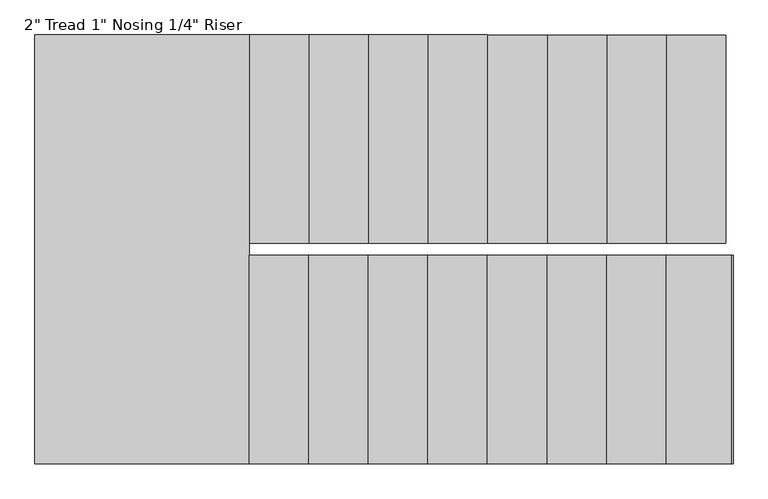
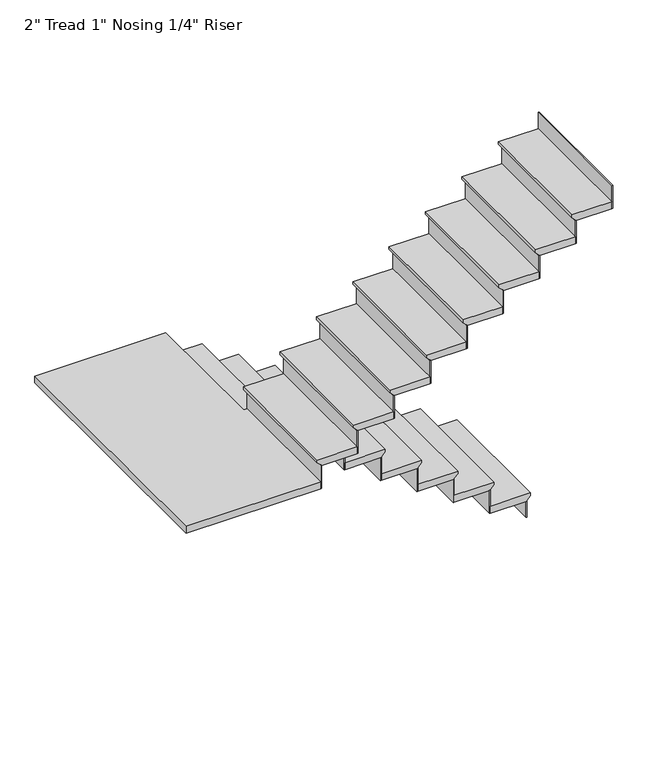
"""IFC4 building model written with IfcOpenShell, lengths in millimetres: stair flight geometry."""

from ifc_helpers import new_model, si_unit, origin, place, context, project, spatial, faceted_brep, source, transform, mapped, element, save


def stair_flight_80fd211d(model_context):
    return source(origin(), model_context, "Body", "Brep", [
        faceted_brep([(-2748.0012202, 5930.6309003, 3198.2833333), (-2748.0012202, 5930.6309003, 3217.3333333), (-2748.0012202, 5041.6309003, 3217.3333333), (-2748.0012202, 5041.6309003, 3198.2833333), (-2773.4012202, 5930.6309003, 3172.8833333), (-2773.4012202, 5041.6309003, 3172.8833333), (-3027.4012202, 5930.6309003, 3217.3333333), (-3027.4012202, 5041.6309003, 3217.3333333), (-2773.4012202, 5041.6309003, 3166.5333333), (-3027.4012202, 5041.6309003, 3166.5333333), (-3027.4012202, 5930.6309003, 3166.5333333), (-2773.4012202, 5930.6309003, 3166.5333333)], [[[0, 1, 2, 3]], [[4, 0, 3, 5]], [[2, 1, 6, 7]], [[8, 9, 10, 11]], [[2, 7, 9, 8, 5, 3]], [[8, 11, 4, 5]], [[6, 1, 0, 4, 11, 10]], [[7, 6, 10, 9]]]),
        faceted_brep([(-2773.4012202, 5930.6309003, 3166.5333333), (-2773.4012202, 5930.6309003, 3048.0), (-2779.7512202, 5930.6309003, 3048.0), (-2779.7512202, 5930.6309003, 3166.5333333), (-2773.4012202, 5041.6309003, 3166.5333333), (-2779.7512202, 5041.6309003, 3166.5333333), (-2779.7512202, 5041.6309003, 3048.0), (-2773.4012202, 5041.6309003, 3048.0)], [[[0, 1, 2, 3]], [[4, 5, 6, 7]], [[1, 0, 4, 7]], [[2, 1, 7, 6]], [[3, 2, 6, 5]], [[0, 3, 5, 4]]]),
        faceted_brep([(-3027.4012202, 5930.6309003, 3335.8666667), (-3027.4012202, 5930.6309003, 3166.5333333), (-3033.7512202, 5930.6309003, 3166.5333333), (-3033.7512202, 5930.6309003, 3335.8666667), (-3027.4012202, 5041.6309003, 3335.8666667), (-3033.7512202, 5041.6309003, 3335.8666667), (-3033.7512202, 5041.6309003, 3166.5333333), (-3027.4012202, 5041.6309003, 3166.5333333)], [[[0, 1, 2, 3]], [[4, 5, 6, 7]], [[1, 0, 4, 7]], [[2, 1, 7, 6]], [[3, 2, 6, 5]], [[0, 3, 5, 4]]]),
        faceted_brep([(-3002.0012202, 5041.6309003, 3386.6666667), (-3002.0012202, 5930.6309003, 3386.6666667), (-3281.4012202, 5930.6309003, 3386.6666667), (-3281.4012202, 5041.6309003, 3386.6666667), (-3027.4012202, 5041.6309003, 3335.8666667), (-3281.4012202, 5041.6309003, 3335.8666667), (-3281.4012202, 5930.6309003, 3335.8666667), (-3027.4012202, 5930.6309003, 3335.8666667), (-3027.4012202, 5041.6309003, 3342.2166667), (-3002.0012202, 5041.6309003, 3367.6166667), (-3027.4012202, 5930.6309003, 3342.2166667), (-3002.0012202, 5930.6309003, 3367.6166667)], [[[0, 1, 2, 3]], [[4, 5, 6, 7]], [[0, 3, 5, 4, 8, 9]], [[4, 7, 10, 8]], [[2, 1, 11, 10, 7, 6]], [[3, 2, 6, 5]], [[11, 1, 0, 9]], [[10, 11, 9, 8]]]),
        faceted_brep([(-3281.4012202, 5930.6309003, 3505.2), (-3281.4012202, 5930.6309003, 3335.8666667), (-3287.7512202, 5930.6309003, 3335.8666667), (-3287.7512202, 5930.6309003, 3505.2), (-3281.4012202, 5041.6309003, 3505.2), (-3287.7512202, 5041.6309003, 3505.2), (-3287.7512202, 5041.6309003, 3335.8666667), (-3281.4012202, 5041.6309003, 3335.8666667)], [[[0, 1, 2, 3]], [[4, 5, 6, 7]], [[1, 0, 4, 7]], [[2, 1, 7, 6]], [[3, 2, 6, 5]], [[0, 3, 5, 4]]]),
        faceted_brep([(-3256.0012202, 5041.6309003, 3556.0), (-3256.0012202, 5930.6309003, 3556.0), (-3535.4012202, 5930.6309003, 3556.0), (-3535.4012202, 5041.6309003, 3556.0), (-3281.4012202, 5041.6309003, 3505.2), (-3535.4012202, 5041.6309003, 3505.2), (-3535.4012202, 5930.6309003, 3505.2), (-3281.4012202, 5930.6309003, 3505.2), (-3281.4012202, 5041.6309003, 3511.55), (-3256.0012202, 5041.6309003, 3536.95), (-3281.4012202, 5930.6309003, 3511.55), (-3256.0012202, 5930.6309003, 3536.95)], [[[0, 1, 2, 3]], [[4, 5, 6, 7]], [[0, 3, 5, 4, 8, 9]], [[4, 7, 10, 8]], [[2, 1, 11, 10, 7, 6]], [[3, 2, 6, 5]], [[11, 1, 0, 9]], [[10, 11, 9, 8]]]),
        faceted_brep([(-3535.4012202, 5930.6309003, 3674.5333333), (-3535.4012202, 5930.6309003, 3505.2), (-3541.7512202, 5930.6309003, 3505.2), (-3541.7512202, 5930.6309003, 3674.5333333), (-3535.4012202, 5041.6309003, 3674.5333333), (-3541.7512202, 5041.6309003, 3674.5333333), (-3541.7512202, 5041.6309003, 3505.2), (-3535.4012202, 5041.6309003, 3505.2)], [[[0, 1, 2, 3]], [[4, 5, 6, 7]], [[1, 0, 4, 7]], [[2, 1, 7, 6]], [[3, 2, 6, 5]], [[0, 3, 5, 4]]]),
        faceted_brep([(-3510.0012202, 5041.6309003, 3725.3333333), (-3510.0012202, 5930.6309003, 3725.3333333), (-3789.4012202, 5930.6309003, 3725.3333333), (-3789.4012202, 5041.6309003, 3725.3333333), (-3535.4012202, 5041.6309003, 3674.5333333), (-3789.4012202, 5041.6309003, 3674.5333333), (-3789.4012202, 5930.6309003, 3674.5333333), (-3535.4012202, 5930.6309003, 3674.5333333), (-3535.4012202, 5041.6309003, 3680.8833333), (-3510.0012202, 5041.6309003, 3706.2833333), (-3535.4012202, 5930.6309003, 3680.8833333), (-3510.0012202, 5930.6309003, 3706.2833333)], [[[0, 1, 2, 3]], [[4, 5, 6, 7]], [[0, 3, 5, 4, 8, 9]], [[4, 7, 10, 8]], [[2, 1, 11, 10, 7, 6]], [[3, 2, 6, 5]], [[11, 1, 0, 9]], [[10, 11, 9, 8]]]),
        faceted_brep([(-3789.4012202, 5930.6309003, 3843.8666667), (-3789.4012202, 5930.6309003, 3674.5333333), (-3795.7512202, 5930.6309003, 3674.5333333), (-3795.7512202, 5930.6309003, 3843.8666667), (-3789.4012202, 5041.6309003, 3843.8666667), (-3795.7512202, 5041.6309003, 3843.8666667), (-3795.7512202, 5041.6309003, 3674.5333333), (-3789.4012202, 5041.6309003, 3674.5333333)], [[[0, 1, 2, 3]], [[4, 5, 6, 7]], [[1, 0, 4, 7]], [[2, 1, 7, 6]], [[3, 2, 6, 5]], [[0, 3, 5, 4]]]),
        faceted_brep([(-3764.0012202, 5041.6309003, 3894.6666667), (-3764.0012202, 5930.6309003, 3894.6666667), (-4043.4012202, 5930.6309003, 3894.6666667), (-4043.4012202, 5041.6309003, 3894.6666667), (-3789.4012202, 5041.6309003, 3843.8666667), (-4043.4012202, 5041.6309003, 3843.8666667), (-4043.4012202, 5930.6309003, 3843.8666667), (-3789.4012202, 5930.6309003, 3843.8666667), (-3789.4012202, 5041.6309003, 3850.2166667), (-3764.0012202, 5041.6309003, 3875.6166667), (-3789.4012202, 5930.6309003, 3850.2166667), (-3764.0012202, 5930.6309003, 3875.6166667)], [[[0, 1, 2, 3]], [[4, 5, 6, 7]], [[0, 3, 5, 4, 8, 9]], [[4, 7, 10, 8]], [[2, 1, 11, 10, 7, 6]], [[3, 2, 6, 5]], [[11, 1, 0, 9]], [[10, 11, 9, 8]]]),
        faceted_brep([(-4043.4012202, 5930.6309003, 4013.2), (-4043.4012202, 5930.6309003, 3843.8666667), (-4049.7512202, 5930.6309003, 3843.8666667), (-4049.7512202, 5930.6309003, 4013.2), (-4043.4012202, 5041.6309003, 4013.2), (-4049.7512202, 5041.6309003, 4013.2), (-4049.7512202, 5041.6309003, 3843.8666667), (-4043.4012202, 5041.6309003, 3843.8666667)], [[[0, 1, 2, 3]], [[4, 5, 6, 7]], [[1, 0, 4, 7]], [[2, 1, 7, 6]], [[3, 2, 6, 5]], [[0, 3, 5, 4]]]),
        faceted_brep([(-4018.0012202, 5041.6309003, 4064.0), (-4018.0012202, 5930.6309003, 4064.0), (-4297.4012202, 5930.6309003, 4064.0), (-4297.4012202, 5041.6309003, 4064.0), (-4043.4012202, 5041.6309003, 4013.2), (-4297.4012202, 5041.6309003, 4013.2), (-4297.4012202, 5930.6309003, 4013.2), (-4043.4012202, 5930.6309003, 4013.2), (-4043.4012202, 5041.6309003, 4019.55), (-4018.0012202, 5041.6309003, 4044.95), (-4043.4012202, 5930.6309003, 4019.55), (-4018.0012202, 5930.6309003, 4044.95)], [[[0, 1, 2, 3]], [[4, 5, 6, 7]], [[0, 3, 5, 4, 8, 9]], [[4, 7, 10, 8]], [[2, 1, 11, 10, 7, 6]], [[3, 2, 6, 5]], [[11, 1, 0, 9]], [[10, 11, 9, 8]]]),
        faceted_brep([(-4297.4012202, 5930.6309003, 4182.5333333), (-4297.4012202, 5930.6309003, 4013.2), (-4303.7512202, 5930.6309003, 4013.2), (-4303.7512202, 5930.6309003, 4182.5333333), (-4297.4012202, 5041.6309003, 4182.5333333), (-4303.7512202, 5041.6309003, 4182.5333333), (-4303.7512202, 5041.6309003, 4013.2), (-4297.4012202, 5041.6309003, 4013.2)], [[[0, 1, 2, 3]], [[4, 5, 6, 7]], [[1, 0, 4, 7]], [[2, 1, 7, 6]], [[3, 2, 6, 5]], [[0, 3, 5, 4]]]),
        faceted_brep([(-4272.0012202, 5041.6309003, 4233.3333333), (-4272.0012202, 5930.6309003, 4233.3333333), (-4551.4012202, 5930.6309003, 4233.3333333), (-4551.4012202, 5041.6309003, 4233.3333333), (-4297.4012202, 5041.6309003, 4182.5333333), (-4551.4012202, 5041.6309003, 4182.5333333), (-4551.4012202, 5930.6309003, 4182.5333333), (-4297.4012202, 5930.6309003, 4182.5333333), (-4297.4012202, 5041.6309003, 4188.8833333), (-4272.0012202, 5041.6309003, 4214.2833333), (-4297.4012202, 5930.6309003, 4188.8833333), (-4272.0012202, 5930.6309003, 4214.2833333)], [[[0, 1, 2, 3]], [[4, 5, 6, 7]], [[0, 3, 5, 4, 8, 9]], [[4, 7, 10, 8]], [[2, 1, 11, 10, 7, 6]], [[3, 2, 6, 5]], [[11, 1, 0, 9]], [[10, 11, 9, 8]]]),
        faceted_brep([(-4551.4012202, 5930.6309003, 4351.8666667), (-4551.4012202, 5930.6309003, 4182.5333333), (-4557.7512202, 5930.6309003, 4182.5333333), (-4557.7512202, 5930.6309003, 4351.8666667), (-4551.4012202, 5041.6309003, 4351.8666667), (-4557.7512202, 5041.6309003, 4351.8666667), (-4557.7512202, 5041.6309003, 4182.5333333), (-4551.4012202, 5041.6309003, 4182.5333333)], [[[0, 1, 2, 3]], [[4, 5, 6, 7]], [[1, 0, 4, 7]], [[2, 1, 7, 6]], [[3, 2, 6, 5]], [[0, 3, 5, 4]]]),
        faceted_brep([(-4526.0012202, 5041.6309003, 4402.6666667), (-4526.0012202, 5930.6309003, 4402.6666667), (-4805.4012202, 5930.6309003, 4402.6666667), (-4805.4012202, 5041.6309003, 4402.6666667), (-4551.4012202, 5041.6309003, 4351.8666667), (-4805.4012202, 5041.6309003, 4351.8666667), (-4805.4012202, 5930.6309003, 4351.8666667), (-4551.4012202, 5930.6309003, 4351.8666667), (-4551.4012202, 5041.6309003, 4358.2166667), (-4526.0012202, 5041.6309003, 4383.6166667), (-4551.4012202, 5930.6309003, 4358.2166667), (-4526.0012202, 5930.6309003, 4383.6166667)], [[[0, 1, 2, 3]], [[4, 5, 6, 7]], [[0, 3, 5, 4, 8, 9]], [[4, 7, 10, 8]], [[2, 1, 11, 10, 7, 6]], [[3, 2, 6, 5]], [[11, 1, 0, 9]], [[10, 11, 9, 8]]]),
        faceted_brep([(-4805.4012202, 5930.6309003, 4521.2), (-4805.4012202, 5930.6309003, 4351.8666667), (-4811.7512202, 5930.6309003, 4351.8666667), (-4811.7512202, 5930.6309003, 4521.2), (-4805.4012202, 5041.6309003, 4521.2), (-4811.7512202, 5041.6309003, 4521.2), (-4811.7512202, 5041.6309003, 4351.8666667), (-4805.4012202, 5041.6309003, 4351.8666667)], [[[0, 1, 2, 3]], [[4, 5, 6, 7]], [[1, 0, 4, 7]], [[2, 1, 7, 6]], [[3, 2, 6, 5]], [[0, 3, 5, 4]]]),
        faceted_brep([(-4754.6012202, 4990.8309003, 4572.0), (-4780.0012202, 4990.8309003, 4572.0), (-4780.0012202, 5930.6309003, 4572.0), (-5694.4012202, 5930.6309003, 4572.0), (-5694.4012202, 4101.8309003, 4572.0), (-4754.6012202, 4101.8309003, 4572.0), (-4780.0012202, 4990.8309003, 4521.2), (-4754.6012202, 4990.8309003, 4521.2), (-4754.6012202, 4101.8309003, 4521.2), (-5694.4012202, 4101.8309003, 4521.2), (-5694.4012202, 5930.6309003, 4521.2), (-4805.4012202, 5930.6309003, 4521.2), (-4805.4012202, 5041.6309003, 4521.2), (-4780.0012202, 5041.6309003, 4521.2), (-4780.0012202, 5041.6309003, 4552.95), (-4780.0012202, 5930.6309003, 4552.95), (-4805.4012202, 5041.6309003, 4527.55), (-4805.4012202, 5930.6309003, 4527.55)], [[[0, 1, 2, 3, 4, 5]], [[6, 7, 8, 9, 10, 11, 12, 13]], [[1, 0, 7, 6]], [[2, 1, 6, 13, 14, 15]], [[13, 12, 16, 14]], [[12, 11, 17, 16]], [[3, 2, 15, 17, 11, 10]], [[4, 3, 10, 9]], [[5, 4, 9, 8]], [[0, 5, 8, 7]], [[17, 15, 14, 16]]]),
        faceted_brep([(-4754.6012202, 4101.8309003, 4690.5333333), (-4754.6012202, 4101.8309003, 4521.2), (-4748.2512202, 4101.8309003, 4521.2), (-4748.2512202, 4101.8309003, 4690.5333333), (-4754.6012202, 4990.8309003, 4690.5333333), (-4748.2512202, 4990.8309003, 4690.5333333), (-4748.2512202, 4990.8309003, 4521.2), (-4754.6012202, 4990.8309003, 4521.2)], [[[0, 1, 2, 3]], [[4, 5, 6, 7]], [[1, 0, 4, 7]], [[2, 1, 7, 6]], [[3, 2, 6, 5]], [[0, 3, 5, 4]]]),
        faceted_brep([(-4780.0012202, 4990.8309003, 4741.3333333), (-4780.0012202, 4101.8309003, 4741.3333333), (-4500.6012202, 4101.8309003, 4741.3333333), (-4500.6012202, 4990.8309003, 4741.3333333), (-4754.6012202, 4990.8309003, 4690.5333333), (-4500.6012202, 4990.8309003, 4690.5333333), (-4500.6012202, 4101.8309003, 4690.5333333), (-4754.6012202, 4101.8309003, 4690.5333333), (-4754.6012202, 4990.8309003, 4696.8833333), (-4780.0012202, 4990.8309003, 4722.2833333), (-4754.6012202, 4101.8309003, 4696.8833333), (-4780.0012202, 4101.8309003, 4722.2833333)], [[[0, 1, 2, 3]], [[4, 5, 6, 7]], [[0, 3, 5, 4, 8, 9]], [[4, 7, 10, 8]], [[2, 1, 11, 10, 7, 6]], [[3, 2, 6, 5]], [[11, 1, 0, 9]], [[10, 11, 9, 8]]]),
        faceted_brep([(-4500.6012202, 4101.8309003, 4859.8666667), (-4500.6012202, 4101.8309003, 4690.5333333), (-4494.2512202, 4101.8309003, 4690.5333333), (-4494.2512202, 4101.8309003, 4859.8666667), (-4500.6012202, 4990.8309003, 4859.8666667), (-4494.2512202, 4990.8309003, 4859.8666667), (-4494.2512202, 4990.8309003, 4690.5333333), (-4500.6012202, 4990.8309003, 4690.5333333)], [[[0, 1, 2, 3]], [[4, 5, 6, 7]], [[1, 0, 4, 7]], [[2, 1, 7, 6]], [[3, 2, 6, 5]], [[0, 3, 5, 4]]]),
        faceted_brep([(-4526.0012202, 4990.8309003, 4910.6666667), (-4526.0012202, 4101.8309003, 4910.6666667), (-4246.6012202, 4101.8309003, 4910.6666667), (-4246.6012202, 4990.8309003, 4910.6666667), (-4500.6012202, 4990.8309003, 4859.8666667), (-4246.6012202, 4990.8309003, 4859.8666667), (-4246.6012202, 4101.8309003, 4859.8666667), (-4500.6012202, 4101.8309003, 4859.8666667), (-4500.6012202, 4990.8309003, 4866.2166667), (-4526.0012202, 4990.8309003, 4891.6166667), (-4500.6012202, 4101.8309003, 4866.2166667), (-4526.0012202, 4101.8309003, 4891.6166667)], [[[0, 1, 2, 3]], [[4, 5, 6, 7]], [[0, 3, 5, 4, 8, 9]], [[4, 7, 10, 8]], [[2, 1, 11, 10, 7, 6]], [[3, 2, 6, 5]], [[11, 1, 0, 9]], [[10, 11, 9, 8]]]),
        faceted_brep([(-4246.6012202, 4101.8309003, 5029.2), (-4246.6012202, 4101.8309003, 4859.8666667), (-4240.2512202, 4101.8309003, 4859.8666667), (-4240.2512202, 4101.8309003, 5029.2), (-4246.6012202, 4990.8309003, 5029.2), (-4240.2512202, 4990.8309003, 5029.2), (-4240.2512202, 4990.8309003, 4859.8666667), (-4246.6012202, 4990.8309003, 4859.8666667)], [[[0, 1, 2, 3]], [[4, 5, 6, 7]], [[1, 0, 4, 7]], [[2, 1, 7, 6]], [[3, 2, 6, 5]], [[0, 3, 5, 4]]]),
        faceted_brep([(-4272.0012202, 4990.8309003, 5080.0), (-4272.0012202, 4101.8309003, 5080.0), (-3992.6012202, 4101.8309003, 5080.0), (-3992.6012202, 4990.8309003, 5080.0), (-4246.6012202, 4990.8309003, 5029.2), (-3992.6012202, 4990.8309003, 5029.2), (-3992.6012202, 4101.8309003, 5029.2), (-4246.6012202, 4101.8309003, 5029.2), (-4246.6012202, 4990.8309003, 5035.55), (-4272.0012202, 4990.8309003, 5060.95), (-4246.6012202, 4101.8309003, 5035.55), (-4272.0012202, 4101.8309003, 5060.95)], [[[0, 1, 2, 3]], [[4, 5, 6, 7]], [[0, 3, 5, 4, 8, 9]], [[4, 7, 10, 8]], [[2, 1, 11, 10, 7, 6]], [[3, 2, 6, 5]], [[11, 1, 0, 9]], [[10, 11, 9, 8]]]),
        faceted_brep([(-3992.6012202, 4101.8309003, 5198.5333333), (-3992.6012202, 4101.8309003, 5029.2), (-3986.2512202, 4101.8309003, 5029.2), (-3986.2512202, 4101.8309003, 5198.5333333), (-3992.6012202, 4990.8309003, 5198.5333333), (-3986.2512202, 4990.8309003, 5198.5333333), (-3986.2512202, 4990.8309003, 5029.2), (-3992.6012202, 4990.8309003, 5029.2)], [[[0, 1, 2, 3]], [[4, 5, 6, 7]], [[1, 0, 4, 7]], [[2, 1, 7, 6]], [[3, 2, 6, 5]], [[0, 3, 5, 4]]]),
        faceted_brep([(-4018.0012202, 4990.8309003, 5249.3333333), (-4018.0012202, 4101.8309003, 5249.3333333), (-3738.6012202, 4101.8309003, 5249.3333333), (-3738.6012202, 4990.8309003, 5249.3333333), (-3992.6012202, 4990.8309003, 5198.5333333), (-3738.6012202, 4990.8309003, 5198.5333333), (-3738.6012202, 4101.8309003, 5198.5333333), (-3992.6012202, 4101.8309003, 5198.5333333), (-3992.6012202, 4990.8309003, 5204.8833333), (-4018.0012202, 4990.8309003, 5230.2833333), (-3992.6012202, 4101.8309003, 5204.8833333), (-4018.0012202, 4101.8309003, 5230.2833333)], [[[0, 1, 2, 3]], [[4, 5, 6, 7]], [[0, 3, 5, 4, 8, 9]], [[4, 7, 10, 8]], [[2, 1, 11, 10, 7, 6]], [[3, 2, 6, 5]], [[11, 1, 0, 9]], [[10, 11, 9, 8]]]),
        faceted_brep([(-3738.6012202, 4101.8309003, 5367.8666667), (-3738.6012202, 4101.8309003, 5198.5333333), (-3732.2512202, 4101.8309003, 5198.5333333), (-3732.2512202, 4101.8309003, 5367.8666667), (-3738.6012202, 4990.8309003, 5367.8666667), (-3732.2512202, 4990.8309003, 5367.8666667), (-3732.2512202, 4990.8309003, 5198.5333333), (-3738.6012202, 4990.8309003, 5198.5333333)], [[[0, 1, 2, 3]], [[4, 5, 6, 7]], [[1, 0, 4, 7]], [[2, 1, 7, 6]], [[3, 2, 6, 5]], [[0, 3, 5, 4]]]),
        faceted_brep([(-3764.0012202, 4990.8309003, 5418.6666667), (-3764.0012202, 4101.8309003, 5418.6666667), (-3484.6012202, 4101.8309003, 5418.6666667), (-3484.6012202, 4990.8309003, 5418.6666667), (-3738.6012202, 4990.8309003, 5367.8666667), (-3484.6012202, 4990.8309003, 5367.8666667), (-3484.6012202, 4101.8309003, 5367.8666667), (-3738.6012202, 4101.8309003, 5367.8666667), (-3738.6012202, 4990.8309003, 5374.2166667), (-3764.0012202, 4990.8309003, 5399.6166667), (-3738.6012202, 4101.8309003, 5374.2166667), (-3764.0012202, 4101.8309003, 5399.6166667)], [[[0, 1, 2, 3]], [[4, 5, 6, 7]], [[0, 3, 5, 4, 8, 9]], [[4, 7, 10, 8]], [[2, 1, 11, 10, 7, 6]], [[3, 2, 6, 5]], [[11, 1, 0, 9]], [[10, 11, 9, 8]]]),
        faceted_brep([(-3484.6012202, 4101.8309003, 5537.2), (-3484.6012202, 4101.8309003, 5367.8666667), (-3478.2512202, 4101.8309003, 5367.8666667), (-3478.2512202, 4101.8309003, 5537.2), (-3484.6012202, 4990.8309003, 5537.2), (-3478.2512202, 4990.8309003, 5537.2), (-3478.2512202, 4990.8309003, 5367.8666667), (-3484.6012202, 4990.8309003, 5367.8666667)], [[[0, 1, 2, 3]], [[4, 5, 6, 7]], [[1, 0, 4, 7]], [[2, 1, 7, 6]], [[3, 2, 6, 5]], [[0, 3, 5, 4]]]),
        faceted_brep([(-3510.0012202, 4990.8309003, 5588.0), (-3510.0012202, 4101.8309003, 5588.0), (-3230.6012202, 4101.8309003, 5588.0), (-3230.6012202, 4990.8309003, 5588.0), (-3484.6012202, 4990.8309003, 5537.2), (-3230.6012202, 4990.8309003, 5537.2), (-3230.6012202, 4101.8309003, 5537.2), (-3484.6012202, 4101.8309003, 5537.2), (-3484.6012202, 4990.8309003, 5543.55), (-3510.0012202, 4990.8309003, 5568.95), (-3484.6012202, 4101.8309003, 5543.55), (-3510.0012202, 4101.8309003, 5568.95)], [[[0, 1, 2, 3]], [[4, 5, 6, 7]], [[0, 3, 5, 4, 8, 9]], [[4, 7, 10, 8]], [[2, 1, 11, 10, 7, 6]], [[3, 2, 6, 5]], [[11, 1, 0, 9]], [[10, 11, 9, 8]]]),
        faceted_brep([(-3230.6012202, 4101.8309003, 5706.5333333), (-3230.6012202, 4101.8309003, 5537.2), (-3224.2512202, 4101.8309003, 5537.2), (-3224.2512202, 4101.8309003, 5706.5333333), (-3230.6012202, 4990.8309003, 5706.5333333), (-3224.2512202, 4990.8309003, 5706.5333333), (-3224.2512202, 4990.8309003, 5537.2), (-3230.6012202, 4990.8309003, 5537.2)], [[[0, 1, 2, 3]], [[4, 5, 6, 7]], [[1, 0, 4, 7]], [[2, 1, 7, 6]], [[3, 2, 6, 5]], [[0, 3, 5, 4]]]),
        faceted_brep([(-3256.0012202, 4990.8309003, 5757.3333333), (-3256.0012202, 4101.8309003, 5757.3333333), (-2976.6012202, 4101.8309003, 5757.3333333), (-2976.6012202, 4990.8309003, 5757.3333333), (-3230.6012202, 4990.8309003, 5706.5333333), (-2976.6012202, 4990.8309003, 5706.5333333), (-2976.6012202, 4101.8309003, 5706.5333333), (-3230.6012202, 4101.8309003, 5706.5333333), (-3230.6012202, 4990.8309003, 5712.8833333), (-3256.0012202, 4990.8309003, 5738.2833333), (-3230.6012202, 4101.8309003, 5712.8833333), (-3256.0012202, 4101.8309003, 5738.2833333)], [[[0, 1, 2, 3]], [[4, 5, 6, 7]], [[0, 3, 5, 4, 8, 9]], [[4, 7, 10, 8]], [[2, 1, 11, 10, 7, 6]], [[3, 2, 6, 5]], [[11, 1, 0, 9]], [[10, 11, 9, 8]]]),
        faceted_brep([(-2976.6012202, 4101.8309003, 5875.8666667), (-2976.6012202, 4101.8309003, 5706.5333333), (-2970.2512202, 4101.8309003, 5706.5333333), (-2970.2512202, 4101.8309003, 5875.8666667), (-2976.6012202, 4990.8309003, 5875.8666667), (-2970.2512202, 4990.8309003, 5875.8666667), (-2970.2512202, 4990.8309003, 5706.5333333), (-2976.6012202, 4990.8309003, 5706.5333333)], [[[0, 1, 2, 3]], [[4, 5, 6, 7]], [[1, 0, 4, 7]], [[2, 1, 7, 6]], [[3, 2, 6, 5]], [[0, 3, 5, 4]]]),
        faceted_brep([(-2722.6012202, 4101.8309003, 6045.2), (-2722.6012202, 4101.8309003, 5875.8666667), (-2716.2512202, 4101.8309003, 5875.8666667), (-2716.2512202, 4101.8309003, 6045.2), (-2722.6012202, 4990.8309003, 6045.2), (-2716.2512202, 4990.8309003, 6045.2), (-2716.2512202, 4990.8309003, 5875.8666667), (-2722.6012202, 4990.8309003, 5875.8666667)], [[[0, 1, 2, 3]], [[4, 5, 6, 7]], [[1, 0, 4, 7]], [[2, 1, 7, 6]], [[3, 2, 6, 5]], [[0, 3, 5, 4]]]),
        faceted_brep([(-3002.0012202, 4990.8309003, 5926.6666667), (-3002.0012202, 4101.8309003, 5926.6666667), (-2722.6012202, 4101.8309003, 5926.6666667), (-2722.6012202, 4990.8309003, 5926.6666667), (-2976.6012202, 4990.8309003, 5875.8666667), (-2722.6012202, 4990.8309003, 5875.8666667), (-2722.6012202, 4101.8309003, 5875.8666667), (-2976.6012202, 4101.8309003, 5875.8666667), (-2976.6012202, 4990.8309003, 5882.2166667), (-3002.0012202, 4990.8309003, 5907.6166667), (-2976.6012202, 4101.8309003, 5882.2166667), (-3002.0012202, 4101.8309003, 5907.6166667)], [[[0, 1, 2, 3]], [[4, 5, 6, 7]], [[0, 3, 5, 4, 8, 9]], [[4, 7, 10, 8]], [[2, 1, 11, 10, 7, 6]], [[3, 2, 6, 5]], [[11, 1, 0, 9]], [[10, 11, 9, 8]]]),
    ])


if __name__ == "__main__":
    model = new_model("IFC4")
    model_context = context("Model", 3, world=origin())
    ifc_project = project(units=[si_unit("LENGTHUNIT", "METRE", prefix="MILLI")], contexts=[model_context])
    site = spatial("IfcSite", under=ifc_project)
    building = spatial("IfcBuilding", under=site)
    placement = place(None, origin())
    stair_flight_shape = stair_flight_80fd211d(model_context)
    element("IfcStairFlight", 1, ObjectType="2\" Tread 1\" Nosing 1/4\" Riser", at=placement, inside=building, context=model_context, shape_type="MappedRepresentation", body=[
        mapped(stair_flight_shape, transform((0.0, 0.0, 0.0), x_axis=(1.0, 0.0, 0.0), y_axis=(0.0, 1.0, 0.0), z_axis=(0.0, 0.0, 1.0))),
    ])
    save(model, "model.ifc")
